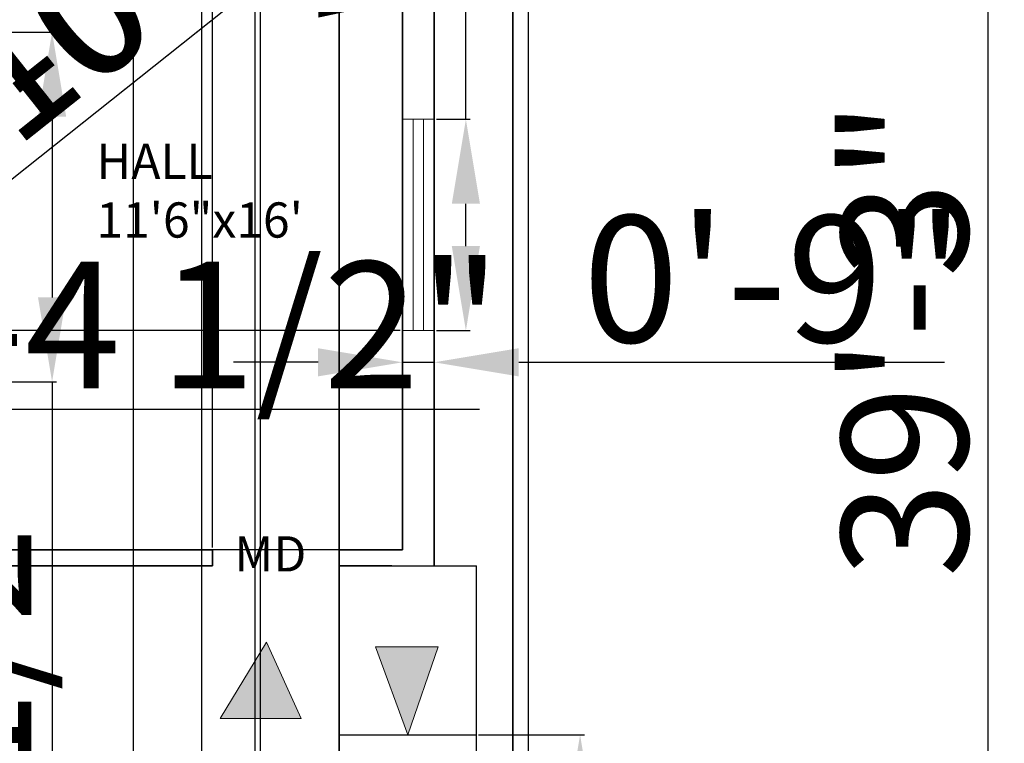
# Model space of a CAD drawing. Units: inches. Extents: x 1041 to 1781, y -140 to 732.
# Tile 3 of 6: x 1359 to 1638, y 153 to 358. Entities that reach past the tile are written whole.
import ezdxf

# ---------------------------------------------------------------- set-up
doc = ezdxf.new("R2010")
doc.units = ezdxf.units.IN
for name, color, linetype, lineweight in [('A-ANNO-SYMB', 7, 'Continuous', 18), ('A-ANNO-TEXT', 7, 'Continuous', 18), ('A-AREA-IDEN', 7, 'Continuous', 20), ('A-FLOR', 7, 'Continuous', 25), ('A-FLOR-STRS', 7, 'Continuous', 25), ('A-GLAZ', 4, 'Continuous', 18), ('A-WALL', 7, 'Continuous', 35), ('C-PROP', 3, 'Continuous', 25), ('dimension', 130, 'Continuous', 18)]:
    doc.layers.add(name, color=color, linetype=linetype, lineweight=lineweight)
doc.layers.add('A-ANNO-SYMB-PATT', color=18, linetype='Continuous', lineweight=18, true_color=0x000000)
doc.styles.get("Standard").update_dxf_attribs({"font": 'arial.ttf'})
doc.dimstyles.new('ISO-25', dxfattribs={"dimtxt": 36, "dimasz": 24, "dimexe": 1.25, "dimexo": 0.625, "dimtad": 1, "dimlunit": 4, "dimtxsty": 'Standard', "dimcen": 2.5, "dimadec": 0, "dimazin": 0, "dimtfac": 1, "dimtmove": 0, "dimatfit": 3, "dimfxl": 1, "dimarcsym": 0})

# ---------------------------------------------------------------- blocks, each defined once
blk = doc.blocks.new('windowcc')
for p, q in [((1195.89, 1013.93), (1195.89, 953.93)), ((1198.89, 1013.93), (1198.89, 953.93)), ((1201.89, 953.93), (1201.89, 1013.93)), ((1204.89, 953.93), (1204.89, 1013.93)), ((1195.89, 953.93), (1204.89, 953.93))]:
    blk.add_line(p, q)
blk = doc.blocks.new('windowcc1')
blk.add_line((1204.89, 1013.93), (1195.89, 1013.93))
blk.add_blockref('windowcc', (0, 0))
blk = doc.blocks.new('*D10')
at = {"layer": 'Defpoints', "color": 0, "transparency": 16777216}
for p in [(1174.94, 364.32), (1183.94, 364.32), (1183.94, 360.72)]:
    blk.add_point(p, dxfattribs=at)
at = {"layer": 'dimension', "color": 0, "lineweight": -2, "transparency": 16777216}
for p, q in [((1174.94, 363.69), (1174.94, 359.47)), ((1183.94, 363.69), (1183.94, 359.47)), ((1150.94, 360.72), (1126.94, 360.72)), ((1174.94, 360.72), (1183.94, 360.72)), ((1207.94, 360.72), (1452.63, 360.72))]:
    blk.add_line(p, q, dxfattribs=at)
at = {"layer": 'dimension', "color": 0, "transparency": 16777216}
for points in [[(1150.94, 364.72), (1150.94, 356.72), (1174.94, 360.72)], [(1207.94, 364.72), (1207.94, 356.72), (1183.94, 360.72)]]:
    blk.add_solid(points, dxfattribs=at)
at = {"layer": 'dimension', "color": 0, "transparency": 16777216, "insert": (1342.28, 379.72), "char_height": 36, "attachment_point": 5}
blk.add_mtext('0\'-9" TYP.', dxfattribs=at)
blk = doc.blocks.new('*D13')
at = {"layer": 'Defpoints', "color": 0, "transparency": 16777216}
for p in [(1476.44, 329.99), (1485.44, 329.99), (1476.44, 269.99)]:
    blk.add_point(p, dxfattribs=at)
at = {"layer": 'dimension', "color": 0, "lineweight": -2, "transparency": 16777216}
for p, q in [((1485.44, 329.99), (1485.44, 687.05)), ((1477.06, 329.99), (1486.69, 329.99)), ((1485.44, 293.99), (1485.44, 305.99)), ((1477.06, 269.99), (1486.69, 269.99))]:
    blk.add_line(p, q, dxfattribs=at)
at = {"layer": 'dimension', "color": 0, "transparency": 16777216}
for points in [[(1481.44, 305.99), (1489.44, 305.99), (1485.44, 329.99)], [(1481.44, 293.99), (1489.44, 293.99), (1485.44, 269.99)]]:
    blk.add_solid(points, dxfattribs=at)
at = {"layer": 'dimension', "color": 0, "transparency": 16777216, "insert": (1466.19, 520.52), "char_height": 36, "attachment_point": 5, "rotation": 90}
blk.add_mtext('WINDOW 5\'-0"', dxfattribs=at)
blk = doc.blocks.new('*D14')
at = {"layer": 'Defpoints', "color": 0, "transparency": 16777216}
for p in [(1467.44, 269.99), (1476.44, 269.99), (1476.44, 260.99)]:
    blk.add_point(p, dxfattribs=at)
at = {"layer": 'dimension', "color": 0, "lineweight": -2, "transparency": 16777216}
for p, q in [((1467.44, 269.36), (1467.44, 259.74)), ((1476.44, 269.36), (1476.44, 259.74)), ((1443.44, 260.99), (1419.44, 260.99)), ((1467.44, 260.99), (1476.44, 260.99)), ((1500.44, 260.99), (1621.38, 260.99))]:
    blk.add_line(p, q, dxfattribs=at)
at = {"layer": 'dimension', "color": 0, "transparency": 16777216}
for points in [[(1443.44, 264.99), (1443.44, 256.99), (1467.44, 260.99)], [(1500.44, 264.99), (1500.44, 256.99), (1476.44, 260.99)]]:
    blk.add_solid(points, dxfattribs=at)
at = {"layer": 'dimension', "color": 0, "transparency": 16777216, "insert": (1572.91, 280), "char_height": 36, "attachment_point": 5}
blk.add_mtext('0\'-9"', dxfattribs=at)
blk = doc.blocks.new('*D16')
at = {"layer": 'Defpoints', "color": 0, "transparency": 16777216}
for p in [(1498.75, 503.23), (1633.79, 503.23), (1498.75, 32.23)]:
    blk.add_point(p, dxfattribs=at)
at = {"layer": 'dimension', "color": 0, "lineweight": -2, "transparency": 16777216}
for p, q in [((1499.37, 503.23), (1635.04, 503.23)), ((1633.79, 56.23), (1633.79, 479.23)), ((1499.37, 32.23), (1635.04, 32.23))]:
    blk.add_line(p, q, dxfattribs=at)
at = {"layer": 'dimension', "color": 0, "transparency": 16777216}
for points in [[(1629.79, 479.23), (1637.79, 479.23), (1633.79, 503.23)], [(1629.79, 56.23), (1637.79, 56.23), (1633.79, 32.23)]]:
    blk.add_solid(points, dxfattribs=at)
at = {"layer": 'dimension', "color": 0, "transparency": 16777216, "insert": (1614.78, 267.73), "char_height": 36, "attachment_point": 5, "rotation": 90}
blk.add_mtext('39\'-3"', dxfattribs=at)
blk = doc.blocks.new('*D18')
at = {"layer": 'Defpoints', "color": 0, "transparency": 16777216}
for p in [(1449.44, 541.68), (1413.44, 207.73), (1449.44, 207.73)]:
    blk.add_point(p, dxfattribs=at)
at = {"layer": 'dimension', "color": 0, "lineweight": -2, "transparency": 16777216}
for p, q in [((1413.44, 208.36), (1413.44, 542.93)), ((1449.44, 208.36), (1449.44, 542.93)), ((1389.44, 541.68), (1365.44, 541.68)), ((1413.44, 541.68), (1449.44, 541.68)), ((1473.44, 541.68), (1594.36, 541.68))]:
    blk.add_line(p, q, dxfattribs=at)
at = {"layer": 'dimension', "color": 0, "transparency": 16777216}
for points in [[(1389.44, 545.68), (1389.44, 537.68), (1413.44, 541.68)], [(1473.44, 545.68), (1473.44, 537.68), (1449.44, 541.68)]]:
    blk.add_solid(points, dxfattribs=at)
at = {"layer": 'dimension', "color": 0, "transparency": 16777216, "insert": (1545.9, 560.7), "char_height": 36, "attachment_point": 5}
blk.add_mtext('3\'-0"', dxfattribs=at)
blk = doc.blocks.new('*D19')
at = {"layer": 'Defpoints', "color": 0, "transparency": 16777216}
for p in [(1354.94, 447.73), (1390.94, 447.73), (1390.94, 2.78)]:
    blk.add_point(p, dxfattribs=at)
at = {"layer": 'dimension', "color": 0, "lineweight": -2, "transparency": 16777216}
for p, q in [((1354.94, 447.11), (1354.94, 1.53)), ((1390.94, 447.11), (1390.94, 1.53)), ((1330.94, 2.78), (1306.94, 2.78)), ((1354.94, 2.78), (1390.94, 2.78)), ((1414.94, 2.78), (1535.86, 2.78))]:
    blk.add_line(p, q, dxfattribs=at)
at = {"layer": 'dimension', "color": 0, "transparency": 16777216}
for points in [[(1330.94, 6.78), (1330.94, -1.22), (1354.94, 2.78)], [(1414.94, 6.78), (1414.94, -1.22), (1390.94, 2.78)]]:
    blk.add_solid(points, dxfattribs=at)
at = {"layer": 'dimension', "color": 0, "transparency": 16777216, "insert": (1487.4, 21.8), "char_height": 36, "attachment_point": 5}
blk.add_mtext('3\'-0"', dxfattribs=at)
blk = doc.blocks.new('*D20')
at = {"layer": 'Defpoints', "color": 0, "transparency": 16777216}
for p in [(1425.44, 395.23), (1449.44, 395.23), (1449.44, 2.78)]:
    blk.add_point(p, dxfattribs=at)
at = {"layer": 'dimension', "color": 0, "lineweight": -2, "transparency": 16777216}
for p, q in [((1425.44, 394.61), (1425.44, 1.53)), ((1449.44, 394.61), (1449.44, 1.53)), ((1401.44, 2.78), (1377.44, 2.78)), ((1425.44, 2.78), (1449.44, 2.78)), ((1473.44, 2.78), (1595, 2.78))]:
    blk.add_line(p, q, dxfattribs=at)
at = {"layer": 'dimension', "color": 0, "transparency": 16777216}
for points in [[(1401.44, 6.78), (1401.44, -1.22), (1425.44, 2.78)], [(1473.44, 6.78), (1473.44, -1.22), (1449.44, 2.78)]]:
    blk.add_solid(points, dxfattribs=at)
at = {"layer": 'dimension', "color": 0, "transparency": 16777216, "insert": (1546.22, 21.79), "char_height": 36, "attachment_point": 5}
blk.add_mtext('2\'-0"', dxfattribs=at)
blk = doc.blocks.new('*D21')
at = {"layer": 'Defpoints', "color": 0, "transparency": 16777216}
for p in [(1449.44, 541.68), (1410.44, 41.23), (1449.44, 41.23)]:
    blk.add_point(p, dxfattribs=at)
at = {"layer": 'dimension', "color": 0, "lineweight": -2, "transparency": 16777216}
for p, q in [((1410.44, 41.86), (1410.44, 542.93)), ((1449.44, 41.86), (1449.44, 542.93)), ((1386.44, 541.68), (1362.44, 541.68)), ((1410.44, 541.68), (1449.44, 541.68)), ((1473.44, 541.68), (1594.36, 541.68))]:
    blk.add_line(p, q, dxfattribs=at)
at = {"layer": 'dimension', "color": 0, "transparency": 16777216}
for points in [[(1386.44, 545.68), (1386.44, 537.68), (1410.44, 541.68)], [(1473.44, 545.68), (1473.44, 537.68), (1449.44, 541.68)]]:
    blk.add_solid(points, dxfattribs=at)
at = {"layer": 'dimension', "color": 0, "transparency": 16777216, "insert": (1545.9, 560.7), "char_height": 36, "attachment_point": 5}
blk.add_mtext('3\'-3"', dxfattribs=at)
blk = doc.blocks.new('*D23')
at = {"layer": 'Defpoints', "color": 0, "transparency": 16777216}
for p in [(1302.68, 270.36), (1321, 247.3), (1302.2, 232.37)]:
    blk.add_point(p, dxfattribs=at)
at = {"layer": 'dimension', "color": 0, "lineweight": -2, "transparency": 16777216}
for p, q in [((1321.47, 285.29), (1416.66, 360.9)), ((1320.61, 247.79), (1301.9, 271.34)), ((1283.89, 255.44), (1302.68, 270.36)), ((1301.82, 232.86), (1283.11, 256.41)), ((1265.09, 240.51), (1246.3, 225.58))]:
    blk.add_line(p, q, dxfattribs=at)
at = {"layer": 'dimension', "color": 0, "transparency": 16777216}
for points in [[(1318.99, 288.42), (1323.96, 282.16), (1302.68, 270.36)], [(1262.61, 243.64), (1267.58, 237.38), (1283.89, 255.44)]]:
    blk.add_solid(points, dxfattribs=at)
at = {"layer": 'dimension', "color": 0, "transparency": 16777216, "insert": (1366.64, 345.44), "char_height": 36, "attachment_point": 5, "rotation": 38.4594}
blk.add_mtext('2\'-0"', dxfattribs=at)
blk = doc.blocks.new('*D29')
at = {"layer": 'Defpoints', "color": 0, "transparency": 16777216}
for p in [(1113.8, 269.99), (1467.44, 269.99), (1467.44, 207.73)]:
    blk.add_point(p, dxfattribs=at)
at = {"layer": 'dimension', "color": 0, "lineweight": -2, "transparency": 16777216}
for p, q in [((1113.8, 269.99), (1113.8, 474.82)), ((1466.81, 269.99), (1112.55, 269.99)), ((1113.8, 231.73), (1113.8, 245.99)), ((1466.81, 207.73), (1112.55, 207.73))]:
    blk.add_line(p, q, dxfattribs=at)
at = {"layer": 'dimension', "color": 0, "transparency": 16777216}
for points in [[(1109.8, 245.99), (1117.8, 245.99), (1113.8, 269.99)], [(1109.8, 231.73), (1117.8, 231.73), (1113.8, 207.73)]]:
    blk.add_solid(points, dxfattribs=at)
at = {"layer": 'dimension', "color": 0, "transparency": 16777216, "insert": (1094.56, 384.41), "char_height": 36, "attachment_point": 5, "rotation": 90}
blk.add_mtext('5\'-2 1/2"', dxfattribs=at)
blk = doc.blocks.new('*D31')
at = {"layer": 'Defpoints', "color": 0, "transparency": 16777216}
for p in [(1390.94, 447.73), (1427, 447.73), (1427, 2.78)]:
    blk.add_point(p, dxfattribs=at)
at = {"layer": 'dimension', "color": 0, "lineweight": -2, "transparency": 16777216}
for p, q in [((1390.94, 447.11), (1390.94, 1.53)), ((1427, 447.11), (1427, 1.53)), ((1366.94, 2.78), (1342.94, 2.78)), ((1390.94, 2.78), (1427, 2.78)), ((1451, 2.78), (1571.93, 2.78))]:
    blk.add_line(p, q, dxfattribs=at)
at = {"layer": 'dimension', "color": 0, "transparency": 16777216}
for points in [[(1366.94, 6.78), (1366.94, -1.22), (1390.94, 2.78)], [(1451, 6.78), (1451, -1.22), (1427, 2.78)]]:
    blk.add_solid(points, dxfattribs=at)
at = {"layer": 'dimension', "color": 0, "transparency": 16777216, "insert": (1523.46, 21.8), "char_height": 36, "attachment_point": 5}
blk.add_mtext('3\'-0"', dxfattribs=at)
blk = doc.blocks.new('*D32')
at = {"layer": 'Defpoints', "color": 0, "transparency": 16777216}
for p in [(1236.44, 447.73), (1278.74, 447.73), (1278.74, 2.78)]:
    blk.add_point(p, dxfattribs=at)
at = {"layer": 'dimension', "color": 0, "lineweight": -2, "transparency": 16777216}
for p, q in [((1236.44, 447.11), (1236.44, 1.53)), ((1278.74, 447.11), (1278.74, 1.53)), ((1212.44, 2.78), (1188.44, 2.78)), ((1236.44, 2.78), (1278.74, 2.78)), ((1302.74, 2.78), (1507.55, 2.78))]:
    blk.add_line(p, q, dxfattribs=at)
at = {"layer": 'dimension', "color": 0, "transparency": 16777216}
for points in [[(1212.44, 6.78), (1212.44, -1.22), (1236.44, 2.78)], [(1302.74, 6.78), (1302.74, -1.22), (1278.74, 2.78)]]:
    blk.add_solid(points, dxfattribs=at)
at = {"layer": 'dimension', "color": 0, "transparency": 16777216, "insert": (1417.15, 22.03), "char_height": 36, "attachment_point": 5}
blk.add_mtext('3\'-6 1/2"', dxfattribs=at)
blk = doc.blocks.new('*D33')
at = {"layer": 'Defpoints', "color": 0, "transparency": 16777216}
for p in [(1488.44, 155.23), (1488.44, 65.23), (1517.89, 65.23)]:
    blk.add_point(p, dxfattribs=at)
at = {"layer": 'dimension', "color": 0, "lineweight": -2, "transparency": 16777216}
for p, q in [((1489.06, 155.23), (1519.14, 155.23)), ((1517.89, 131.23), (1517.89, 89.23)), ((1489.06, 65.23), (1519.14, 65.23)), ((1517.89, 65.23), (1517.89, -55.42))]:
    blk.add_line(p, q, dxfattribs=at)
at = {"layer": 'dimension', "color": 0, "transparency": 16777216}
for points in [[(1513.89, 131.23), (1521.89, 131.23), (1517.89, 155.23)], [(1513.89, 89.23), (1521.89, 89.23), (1517.89, 65.23)]]:
    blk.add_solid(points, dxfattribs=at)
at = {"layer": 'dimension', "color": 0, "transparency": 16777216, "insert": (1498.88, -7.09), "char_height": 36, "attachment_point": 5, "rotation": 90}
blk.add_mtext('7\'-6"', dxfattribs=at)
blk = doc.blocks.new('*D35')
at = {"layer": 'Defpoints', "color": 0, "transparency": 16777216}
for p in [(1321.94, 541.68), (1297.94, 165.73), (1321.94, 165.73)]:
    blk.add_point(p, dxfattribs=at)
at = {"layer": 'dimension', "color": 0, "lineweight": -2, "transparency": 16777216}
for p, q in [((1297.94, 166.36), (1297.94, 542.93)), ((1321.94, 166.36), (1321.94, 542.93)), ((1273.94, 541.68), (1249.94, 541.68)), ((1297.94, 541.68), (1321.94, 541.68)), ((1345.94, 541.68), (1467.5, 541.68))]:
    blk.add_line(p, q, dxfattribs=at)
at = {"layer": 'dimension', "color": 0, "transparency": 16777216}
for points in [[(1273.94, 545.68), (1273.94, 537.68), (1297.94, 541.68)], [(1345.94, 545.68), (1345.94, 537.68), (1321.94, 541.68)]]:
    blk.add_solid(points, dxfattribs=at)
at = {"layer": 'dimension', "color": 0, "transparency": 16777216, "insert": (1418.72, 560.69), "char_height": 36, "attachment_point": 5}
blk.add_mtext('2\'-0"', dxfattribs=at)
blk = doc.blocks.new('*D39')
at = {"layer": 'Defpoints', "color": 0, "transparency": 16777216}
for p in [(1467.44, 541.68), (1449.44, 207.73), (1467.44, 207.73)]:
    blk.add_point(p, dxfattribs=at)
at = {"layer": 'dimension', "color": 0, "lineweight": -2, "transparency": 16777216}
for p, q in [((1449.44, 208.36), (1449.44, 542.93)), ((1467.44, 208.36), (1467.44, 542.93)), ((1425.44, 541.68), (1401.44, 541.68)), ((1449.44, 541.68), (1467.44, 541.68)), ((1491.44, 541.68), (1609, 541.68))]:
    blk.add_line(p, q, dxfattribs=at)
at = {"layer": 'dimension', "color": 0, "transparency": 16777216}
for points in [[(1425.44, 545.68), (1425.44, 537.68), (1449.44, 541.68)], [(1491.44, 545.68), (1491.44, 537.68), (1467.44, 541.68)]]:
    blk.add_solid(points, dxfattribs=at)
at = {"layer": 'dimension', "color": 0, "transparency": 16777216, "insert": (1562.22, 560.69), "char_height": 36, "attachment_point": 5}
blk.add_mtext('1\'-6"', dxfattribs=at)
blk = doc.blocks.new('*D43')
at = {"layer": 'Defpoints', "color": 0, "transparency": 16777216}
for p in [(1284.4, 247.68), (1183.94, 218.23), (1284.4, 218.23)]:
    blk.add_point(p, dxfattribs=at)
at = {"layer": 'dimension', "color": 0, "lineweight": -2, "transparency": 16777216}
for p, q in [((1183.94, 218.86), (1183.94, 248.93)), ((1207.94, 247.68), (1260.4, 247.68)), ((1284.4, 218.86), (1284.4, 248.93)), ((1284.4, 247.68), (1489.28, 247.68))]:
    blk.add_line(p, q, dxfattribs=at)
at = {"layer": 'dimension', "color": 0, "transparency": 16777216}
for points in [[(1207.94, 251.68), (1207.94, 243.68), (1183.94, 247.68)], [(1260.4, 251.68), (1260.4, 243.68), (1284.4, 247.68)]]:
    blk.add_solid(points, dxfattribs=at)
at = {"layer": 'dimension', "color": 0, "transparency": 16777216, "insert": (1398.84, 266.92), "char_height": 36, "attachment_point": 5}
blk.add_mtext('8\'-4 1/2"', dxfattribs=at)
blk = doc.blocks.new('*D44')
at = {"layer": 'Defpoints', "color": 0, "transparency": 16777216}
for p in [(1338.44, 354.73), (1338.44, 255.41), (1367.89, 255.41)]:
    blk.add_point(p, dxfattribs=at)
at = {"layer": 'dimension', "color": 0, "lineweight": -2, "transparency": 16777216}
for p, q in [((1339.06, 354.73), (1369.14, 354.73)), ((1367.89, 330.73), (1367.89, 279.41)), ((1339.06, 255.41), (1369.14, 255.41)), ((1367.89, 255.41), (1367.89, 50.53))]:
    blk.add_line(p, q, dxfattribs=at)
at = {"layer": 'dimension', "color": 0, "transparency": 16777216}
for points in [[(1363.89, 330.73), (1371.89, 330.73), (1367.89, 354.73)], [(1363.89, 279.41), (1371.89, 279.41), (1367.89, 255.41)]]:
    blk.add_solid(points, dxfattribs=at)
at = {"layer": 'dimension', "color": 0, "transparency": 16777216, "insert": (1348.64, 140.97), "char_height": 36, "attachment_point": 5, "rotation": 90}
blk.add_mtext('8\'-3 1/2"', dxfattribs=at)
blk = doc.blocks.new('*D45')
at = {"layer": 'Defpoints', "color": 0, "transparency": 16777216}
for p in [(1283.89, 255.44), (1302.2, 232.37), (1284.4, 218.23)]:
    blk.add_point(p, dxfattribs=at)
at = {"layer": 'dimension', "color": 0, "lineweight": -2, "transparency": 16777216}
for p, q in [((1302.68, 270.36), (1482.32, 413.05)), ((1266.08, 241.29), (1283.89, 255.44)), ((1301.82, 232.86), (1283.11, 256.41)), ((1284.01, 218.72), (1265.3, 242.27)), ((1247.29, 226.37), (1228.5, 211.44))]:
    blk.add_line(p, q, dxfattribs=at)
at = {"layer": 'dimension', "color": 0, "transparency": 16777216}
for points in [[(1300.19, 273.49), (1305.17, 267.23), (1283.89, 255.44)], [(1244.8, 229.5), (1249.78, 223.23), (1266.08, 241.29)]]:
    blk.add_solid(points, dxfattribs=at)
at = {"layer": 'dimension', "color": 0, "transparency": 16777216, "insert": (1389.93, 364.23), "char_height": 36, "attachment_point": 5, "rotation": 38.4594}
blk.add_mtext('1\'-10 1/2"', dxfattribs=at)

msp = doc.modelspace()

# ---------------------------------------------------------------- hatches: boundary and pattern name
at = {"layer": 'A-ANNO-SYMB-PATT'}
h = msp.add_hatch(color=256, dxfattribs=at)
h.dxf.hatch_style = 1
h.paths.add_polyline_path([(1428.789, 181.54), (1415.61, 159.812), (1438.673, 159.812)])
h.paths.add_polyline_path([(1477.55, 180.223), (1459.759, 180.223), (1468.938, 155.233)])

# ---------------------------------------------------------------- linework, layer by layer
at = {"layer": 'A-ANNO-SYMB'}
for p, q in [((1428.789, 181.54), (1415.61, 159.812)), ((1438.673, 159.812), (1428.789, 181.54)), ((1459.759, 180.223), (1477.55, 180.223)), ((1468.938, 155.233), (1459.759, 180.223)), ((1477.55, 180.223), (1468.938, 155.233)), ((1415.61, 159.812), (1438.673, 159.812))]:
    msp.add_line(p, q, dxfattribs=at)
at = {"layer": 'A-FLOR'}
for p in [(1464.438, 203.233), (1488.438, 32.233)]:
    msp.add_line(p, (1488.438, 203.233), dxfattribs=at)
at = {"layer": 'A-FLOR-STRS'}
for q in [(1449.438, 41.233), (1488.438, 155.233)]:
    msp.add_line((1449.438, 155.233), q, dxfattribs=at)
at = {"layer": 'A-WALL'}
for p, q in [((1498.749, 32.233), (1498.749, 512.233)), ((1476.438, 203.233), (1476.438, 456.733)), ((1467.438, 207.733), (1467.438, 395.233)), ((1333.938, 207.733), (1413.438, 207.733)), ((1413.438, 207.733), (1413.438, 203.233)), ((1467.438, 207.733), (1449.438, 207.733)), ((1449.438, 207.733), (1449.438, 203.233)), ((1449.438, 207.733), (1467.438, 207.733)), ((1338.438, 203.233), (1413.438, 203.233)), ((1449.438, 203.233), (1464.438, 203.233))]:
    msp.add_line(p, q, dxfattribs=at)
at = {"layer": 'C-PROP'}
msp.add_line((1503.249, 32.233), (1503.249, 512.233), dxfattribs=at)

# ---------------------------------------------------------------- block references
at = {"layer": 'A-GLAZ'}
msp.add_blockref('windowcc1', (271.549, -683.944), dxfattribs=at)

# ---------------------------------------------------------------- texts
at = {"layer": 'A-ANNO-TEXT', "insert": (1419.664, 211.592), "char_height": 10, "attachment_point": 1}
msp.add_mtext_dynamic_manual_height_columns('MD', width=64.5482, gutter_width=12.5, heights=[0], dxfattribs=at)
at = {"layer": 'A-AREA-IDEN', "insert": (1380.458, 323.062), "char_height": 10, "attachment_point": 1}
msp.add_mtext_dynamic_manual_height_columns('HALL\\P11\'6"x16\'', width=64.5482, gutter_width=12.5, heights=[0], dxfattribs=at)

# ---------------------------------------------------------------- dimensions: what is measured, and where the dimension line sits
at = {"layer": 'dimension'}
dim = msp.add_linear_dim(base=(1485.438, 329.99), p1=(1476.438, 269.99), p2=(1476.438, 329.99), angle=90, text='WINDOW <>', dimstyle='ISO-25', override={"dimdec": 1, "dimlfac": 1, "dimrnd": 0, "dimzin": 1, "dimdsep": 46, "dimlunit": 4, "dimfrac": 2}, dxfattribs=at)
dim.commit()
dim.dimension.update_dxf_attribs({"geometry": '*D13', "text_midpoint": (1466.186, 520.519)})
for base, p1, p2, picture, middle in [((1321.938, 541.683), (1297.938, 165.733), (1321.938, 165.733), '*D35', (1418.718, 560.688)), ((1449.438, 541.683), (1410.438, 41.233), (1449.438, 41.233), '*D21', (1545.899, 560.7)), ((1449.438, 541.683), (1413.438, 207.733), (1449.438, 207.733), '*D18', (1545.899, 560.7)), ((1467.438, 541.683), (1449.438, 207.733), (1467.438, 207.733), '*D39', (1562.217, 560.688)), ((1278.743, 2.783), (1236.438, 447.733), (1278.743, 447.733), '*D32', (1417.147, 22.034)), ((1390.938, 2.783), (1354.938, 447.733), (1390.938, 447.733), '*D19', (1487.399, 21.8)), ((1427.003, 2.783), (1390.938, 447.733), (1427.003, 447.733), '*D31', (1523.464, 21.8)), ((1449.438, 2.783), (1425.438, 395.233), (1449.438, 395.233), '*D20', (1546.218, 21.788)), ((1284.399, 247.683), (1183.938, 218.233), (1284.399, 218.233), '*D43', (1398.839, 266.921)), ((1476.438, 260.99), (1467.438, 269.99), (1476.438, 269.99), '*D14', (1572.911, 279.996))]:
    dim = msp.add_linear_dim(base=base, p1=p1, p2=p2, dimstyle='ISO-25', override={"dimdec": 1, "dimlfac": 1, "dimrnd": 0, "dimzin": 1, "dimdsep": 46, "dimlunit": 4, "dimfrac": 2}, dxfattribs=at)
    dim.commit()
    dim.dimension.update_dxf_attribs({"geometry": picture, "text_midpoint": middle})
for base, p1, p2, angle, picture, middle in [((1633.794, 503.233), (1498.749, 32.233), (1498.749, 503.233), 90, '*D16', (1614.777, 267.733)), ((1113.799, 269.99), (1467.438, 207.733), (1467.438, 269.99), 90, '*D29', (1094.56, 384.406)), ((1283.887, 255.436), (1284.399, 218.233), (1302.204, 232.375), 38.45936, '*D45', (1389.932, 364.234)), ((1302.68, 270.363), (1302.204, 232.375), (1320.997, 247.302), 38.45936, '*D23', (1366.644, 345.439)), ((1367.888, 255.408), (1338.438, 354.733), (1338.438, 255.408), 270, '*D44', (1348.636, 140.967)), ((1517.888, 65.233), (1488.438, 155.233), (1488.438, 65.233), 270, '*D33', (1498.882, -7.094))]:
    dim = msp.add_linear_dim(base=base, p1=p1, p2=p2, angle=angle, dimstyle='ISO-25', override={"dimdec": 1, "dimlfac": 1, "dimrnd": 0, "dimzin": 1, "dimdsep": 46, "dimlunit": 4, "dimfrac": 2}, dxfattribs=at)
    dim.commit()
    dim.dimension.update_dxf_attribs({"geometry": picture, "text_midpoint": middle})
dim = msp.add_linear_dim(base=(1183.938, 360.718), p1=(1174.938, 364.318), p2=(1183.938, 364.318), text='<> TYP.', dimstyle='ISO-25', override={"dimdec": 1, "dimlfac": 1, "dimrnd": 0, "dimzin": 1, "dimdsep": 46, "dimlunit": 4, "dimfrac": 2}, dxfattribs=at)
dim.commit()
dim.dimension.update_dxf_attribs({"geometry": '*D10', "text_midpoint": (1342.281, 379.723)})

doc.saveas('drawing.dxf')
